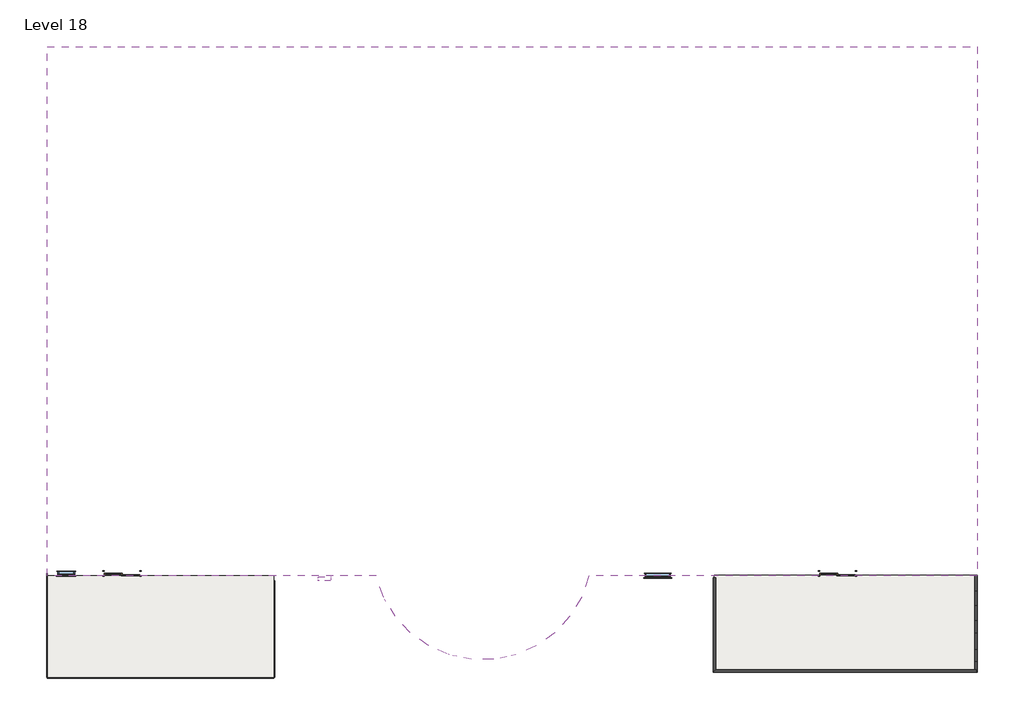
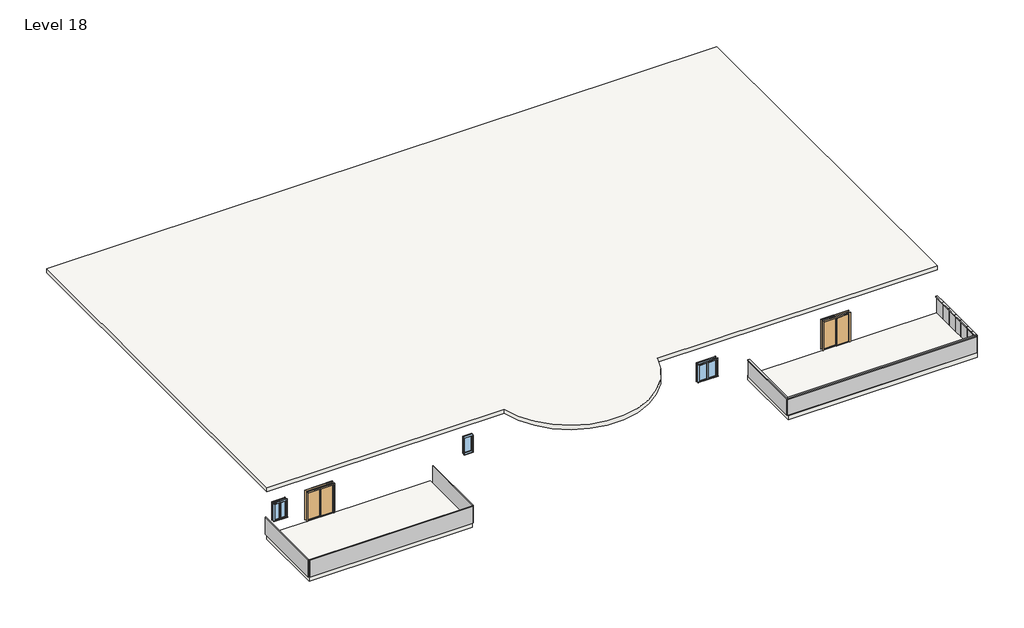
# One storey: 12 plates, 10 members, 3 slabs, 3 windows, 2 doors.
"""IFC4 building model written with IfcOpenShell, lengths in millimetres."""

from ifc_helpers import new_model, si_unit, point, frame, frame_2d, origin, place, context, project, spatial, polyline, circle_curve, trimmed, segment, composite_curve, outline, extrude, transform, mapped, element, save
from components import door_076b30e0, member_47bfaf8a, member_aa870034, member_75074519, member_cae490a4, member_7096a90e, member_cf286210, member_fed80fbc, system_panel_glazed_f269d4c8, system_panel_glazed_7af1c9c3, system_panel_glazed_904ef9a5, system_panel_glazed_078a25c0, system_panel_glazed_c3939aa2, system_panel_glazed_2b5622e6, system_panel_glazed_b96adab1, system_panel_glazed_18441643, system_panel_glazed_400a69f6, window_bb17773d, window_0862ab64, window_80bd9af0

model = new_model("IFC4")

# Units and contexts
model_context = context("Model", 3, world=origin())
ifc_project = project(units=[si_unit("LENGTHUNIT", "METRE", prefix="MILLI")], contexts=[model_context])

# Site, building, storey
site = spatial("IfcSite", under=ifc_project)
building = spatial("IfcBuilding", under=site)
storey = spatial("IfcBuildingStorey", under=building, Name="Level 18", Elevation=29870.4)

# Doors
placement = place(None, origin())
door_shape = door_076b30e0(model_context)
element("IfcDoor", 1, ObjectType="Door-Double-Sliding : 68\" x 80\"", at=placement, inside=storey, context=model_context, shape_type="MappedRepresentation", body=[
    mapped(door_shape, transform((-16191.585279, -12227.7237084, 29870.4), x_axis=(-1.0, 0.0, 0.0), y_axis=(0.0, -1.0, 0.0), z_axis=(0.0, 0.0, 1.0))),
])
element("IfcDoor", 2, ObjectType="Door-Double-Sliding : 68\" x 80\"", at=placement, inside=storey, context=model_context, shape_type="MappedRepresentation", body=[
    mapped(door_shape, transform((18682.614721, -12227.7237084, 29870.4), x_axis=(-1.0, 0.0, 0.0), y_axis=(0.0, -1.0, 0.0), z_axis=(0.0, 0.0, 1.0))),
])

# Members
member_shape = member_47bfaf8a(model_context)
element("IfcMember", 3, ObjectType="Rectangular Mullion : 2.5\" x 5\" rectangular", at=placement, inside=storey, context=model_context, shape_type="MappedRepresentation", body=[
    mapped(member_shape, transform((25445.364721, -15278.1106184, 31089.6), x_axis=(0.0, 0.0, 1.0), y_axis=(-1.0, 0.0, 0.0), z_axis=(0.0, -1.0, 0.0))),
])
element("IfcMember", 4, ObjectType="Rectangular Mullion : 2.5\" x 5\" rectangular", at=placement, inside=storey, context=model_context, shape_type="MappedRepresentation", body=[
    mapped(member_shape, transform((25445.364721, -16649.7106184, 31089.6), x_axis=(0.0, 0.0, 1.0), y_axis=(-1.0, 0.0, 0.0), z_axis=(0.0, -1.0, 0.0))),
])
member_2_shape = member_aa870034(model_context)
element("IfcMember", 5, ObjectType="Rectangular Mullion : 2.5\" x 5\" rectangular", at=placement, inside=storey, context=model_context, shape_type="MappedRepresentation", body=[
    mapped(member_2_shape, transform((25445.364721, -16040.1106184, 31089.6), x_axis=(0.0, 0.0, 1.0), y_axis=(-1.0, 0.0, 0.0), z_axis=(0.0, -1.0, 0.0))),
])
member_3_shape = member_75074519(model_context)
element("IfcMember", 6, ObjectType="Rectangular Mullion : 2.5\" x 5\" rectangular", at=placement, inside=storey, context=model_context, shape_type="MappedRepresentation", body=[
    mapped(member_3_shape, transform((25445.364721, -17106.9106184, 29870.4), x_axis=(0.0, -1.0, 0.0), y_axis=(-1.0, 0.0, 0.0), z_axis=(0.0, 0.0, -1.0))),
])
member_4_shape = member_cae490a4(model_context)
element("IfcMember", 7, ObjectType="Rectangular Mullion : 2.5\" x 5\" rectangular", at=placement, inside=storey, context=model_context, shape_type="MappedRepresentation", body=[
    mapped(member_4_shape, transform((25445.364721, -13193.7193451, 31089.6), x_axis=(0.0, 0.0, 1.0), y_axis=(-1.0, 0.0, 0.0), z_axis=(0.0, -1.0, 0.0))),
])
element("IfcMember", 8, ObjectType="Rectangular Mullion : 2.5\" x 5\" rectangular", at=placement, inside=storey, context=model_context, shape_type="MappedRepresentation", body=[
    mapped(member_4_shape, transform((25445.364721, -13931.1149817, 31089.6), x_axis=(0.0, 0.0, 1.0), y_axis=(-1.0, 0.0, 0.0), z_axis=(0.0, -1.0, 0.0))),
])
element("IfcMember", 9, ObjectType="Rectangular Mullion : 2.5\" x 5\" rectangular", at=placement, inside=storey, context=model_context, shape_type="MappedRepresentation", body=[
    mapped(member_4_shape, transform((25445.364721, -14668.5106184, 31089.6), x_axis=(0.0, 0.0, 1.0), y_axis=(-1.0, 0.0, 0.0), z_axis=(0.0, -1.0, 0.0))),
])
member_5_shape = member_7096a90e(model_context)
element("IfcMember", 10, ObjectType="Rectangular Mullion : 2.5\" x 5\" rectangular", at=placement, inside=storey, context=model_context, shape_type="MappedRepresentation", body=[
    mapped(member_5_shape, transform((25445.364721, -17043.4106184, 31089.6), x_axis=(0.0, 0.0, 1.0), y_axis=(-1.0, 0.0, 0.0), z_axis=(0.0, -1.0, 0.0))),
])
member_6_shape = member_cf286210(model_context)
element("IfcMember", 11, ObjectType="Rectangular Mullion : 2.5\" x 5\" rectangular", at=placement, inside=storey, context=model_context, shape_type="MappedRepresentation", body=[
    mapped(member_6_shape, transform((12687.7364138, -12561.0601244, 31089.6), x_axis=(0.0, 0.0, 1.0), y_axis=(1.0, 0.0, 0.0), z_axis=(0.0, 1.0, 0.0))),
])
member_7_shape = member_fed80fbc(model_context)
element("IfcMember", 12, ObjectType="Rectangular Mullion : 2.5\" x 5\" rectangular", at=placement, inside=storey, context=model_context, shape_type="MappedRepresentation", body=[
    mapped(member_7_shape, transform((12687.7364138, -17106.9106184, 31089.6), x_axis=(0.0, 0.0, 1.0), y_axis=(0.0, 1.0, 0.0), z_axis=(-1.0, 0.0, 0.0))),
])

# Plates
system_panel_glazed_shape = system_panel_glazed_f269d4c8(model_context)
element("IfcPlate", 13, ObjectType="System Panel : Glazed", at=placement, inside=storey, context=model_context, shape_type="MappedRepresentation", body=[
    mapped(system_panel_glazed_shape, transform((25445.364721, -15659.1106184, 29870.4), x_axis=(0.0, -1.0, 0.0), y_axis=(1.0, 0.0, 0.0), z_axis=(0.0, 0.0, 1.0))),
])
system_panel_glazed_2_shape = system_panel_glazed_7af1c9c3(model_context)
element("IfcPlate", 14, ObjectType="System Panel : Glazed", at=placement, inside=storey, context=model_context, shape_type="MappedRepresentation", body=[
    mapped(system_panel_glazed_2_shape, transform((25445.364721, -16344.9106184, 29870.4), x_axis=(0.0, -1.0, 0.0), y_axis=(1.0, 0.0, 0.0), z_axis=(0.0, 0.0, 1.0))),
])
element("IfcPlate", 15, ObjectType="System Panel : Glazed", at=placement, inside=storey, context=model_context, shape_type="MappedRepresentation", body=[
    mapped(system_panel_glazed_2_shape, transform((25445.364721, -14973.3106184, 29870.4), x_axis=(0.0, -1.0, 0.0), y_axis=(1.0, 0.0, 0.0), z_axis=(0.0, 0.0, 1.0))),
])
system_panel_glazed_3_shape = system_panel_glazed_904ef9a5(model_context)
element("IfcPlate", 16, ObjectType="System Panel : Glazed", at=placement, inside=storey, context=model_context, shape_type="MappedRepresentation", body=[
    mapped(system_panel_glazed_3_shape, transform((25445.364721, -12825.0215267, 29870.4), x_axis=(0.0, -1.0, 0.0), y_axis=(1.0, 0.0, 0.0), z_axis=(0.0, 0.0, 1.0))),
])
element("IfcPlate", 17, ObjectType="System Panel : Glazed", at=placement, inside=storey, context=model_context, shape_type="MappedRepresentation", body=[
    mapped(system_panel_glazed_3_shape, transform((25445.364721, -14299.8128001, 29870.4), x_axis=(0.0, -1.0, 0.0), y_axis=(1.0, 0.0, 0.0), z_axis=(0.0, 0.0, 1.0))),
])
element("IfcPlate", 18, ObjectType="System Panel : Glazed", at=placement, inside=storey, context=model_context, shape_type="MappedRepresentation", body=[
    mapped(system_panel_glazed_3_shape, transform((25445.364721, -13562.4171634, 29870.4), x_axis=(0.0, -1.0, 0.0), y_axis=(1.0, 0.0, 0.0), z_axis=(0.0, 0.0, 1.0))),
])
system_panel_glazed_4_shape = system_panel_glazed_078a25c0(model_context)
element("IfcPlate", 19, ObjectType="System Panel : Glazed", at=placement, inside=storey, context=model_context, shape_type="MappedRepresentation", body=[
    mapped(system_panel_glazed_4_shape, transform((19066.5505674, -17106.9106184, 29870.4), x_axis=(-1.0, 0.0, 0.0), y_axis=(0.0, -1.0, 0.0), z_axis=(0.0, 0.0, 1.0))),
])
system_panel_glazed_5_shape = system_panel_glazed_c3939aa2(model_context)
element("IfcPlate", 20, ObjectType="System Panel : Glazed", at=placement, inside=storey, context=model_context, shape_type="MappedRepresentation", body=[
    mapped(system_panel_glazed_5_shape, transform((25445.364721, -16846.5606184, 29870.4), x_axis=(0.0, -1.0, 0.0), y_axis=(1.0, 0.0, 0.0), z_axis=(0.0, 0.0, 1.0))),
])
system_panel_glazed_6_shape = system_panel_glazed_2b5622e6(model_context)
element("IfcPlate", 21, ObjectType="System Panel : Glazed", at=placement, inside=storey, context=model_context, shape_type="MappedRepresentation", body=[
    mapped(system_panel_glazed_6_shape, transform((12687.7364138, -14833.9853714, 29870.4), x_axis=(0.0, 1.0, 0.0), y_axis=(-1.0, 0.0, 0.0), z_axis=(0.0, 0.0, 1.0))),
])
system_panel_glazed_7_shape = system_panel_glazed_b96adab1(model_context)
element("IfcPlate", 22, ObjectType="System Panel : Glazed", at=placement, inside=storey, context=model_context, shape_type="MappedRepresentation", body=[
    mapped(system_panel_glazed_7_shape, transform((-14302.7926538, -17411.944108, 29870.4), x_axis=(-1.0, 0.0, 0.0), y_axis=(0.0, -1.0, 0.0), z_axis=(0.0, 0.0, 1.0))),
])
system_panel_glazed_8_shape = system_panel_glazed_18441643(model_context)
element("IfcPlate", 23, ObjectType="System Panel : Glazed", at=placement, inside=storey, context=model_context, shape_type="MappedRepresentation", body=[
    mapped(system_panel_glazed_8_shape, transform((-19823.785279, -14883.3339082, 29870.4), x_axis=(0.0, 1.0, 0.0), y_axis=(-1.0, 0.0, 0.0), z_axis=(0.0, 0.0, 1.0))),
])
system_panel_glazed_9_shape = system_panel_glazed_400a69f6(model_context)
element("IfcPlate", 24, ObjectType="System Panel : Glazed", at=placement, inside=storey, context=model_context, shape_type="MappedRepresentation", body=[
    mapped(system_panel_glazed_9_shape, transform((-8781.8000285, -15065.3724195, 29870.4), x_axis=(0.0, -1.0, 0.0), y_axis=(1.0, 0.0, 0.0), z_axis=(0.0, 0.0, 1.0))),
])

# Slabs
element("IfcSlab", 25, ObjectType="Generic - 12\"", at=placement, inside=storey, context=model_context, shape_type="SweptSolid", body=[
    extrude(outline(composite_curve([segment(polyline([(25489.814721, 13330.837176), (25489.814721, -12475.562824), (6571.5594464, -12475.562824)]), True, "CONTINUOUS"), segment(trimmed(circle_curve(frame_2d((1385.214721, -11244.9297828)), 5330.3498284), [point((6571.5594464, -12475.562824))], [point((-3801.1300045, -12475.562824))], False, "CARTESIAN"), True, "CONTINUOUS"), segment(polyline([(-3801.1300045, -12475.562824), (-19823.785279, -12475.562824), (-19823.785279, 13330.837176), (25489.814721, 13330.837176)]), True, "CONTINUOUS")], self_intersect=False)), frame((0.0, 0.0, 32956.1464133), z_axis=(0.0, 0.0, 1.0), x_axis=(1.0, 0.0, 0.0)), (0.0, 0.0, 1.0), 304.8),
])
element("IfcSlab", 26, ObjectType="Generic - 12\"", at=placement, inside=storey, context=model_context, shape_type="SweptSolid", body=[
    extrude(outline(polyline([(25489.814721, -12433.6961364), (25489.814721, -17172.4176946), (12687.7364138, -17172.4176946), (12687.7364138, -12433.6961364), (25489.814721, -12433.6961364)])), frame((0.0, 0.0, 29565.6), z_axis=(0.0, 0.0, 1.0), x_axis=(1.0, 0.0, 0.0)), (0.0, 0.0, 1.0), 304.8),
])
element("IfcSlab", 27, ObjectType="Generic - 12\"", at=placement, inside=storey, context=model_context, shape_type="SweptSolid", body=[
    extrude(outline(polyline([(-8781.8000285, -12456.3237084), (-8781.8000285, -17411.944108), (-19823.785279, -17411.944108), (-19823.785279, -12456.3237084), (-8781.8000285, -12456.3237084)])), frame((0.0, 0.0, 29565.6), z_axis=(0.0, 0.0, 1.0), x_axis=(1.0, 0.0, 0.0)), (0.0, 0.0, 1.0), 304.8),
])

# Windows
window_shape = window_bb17773d(model_context)
element("IfcWindow", 28, ObjectType="Casement Dbl with Trim : 32\" x 48\"", at=placement, inside=storey, context=model_context, shape_type="MappedRepresentation", body=[
    mapped(window_shape, transform((-18909.385279, -12335.6737084, 29754.8931655), x_axis=(-1.0, 0.0, 0.0), y_axis=(0.0, -1.0, 0.0), z_axis=(0.0, 0.0, 1.0))),
])
window_2_shape = window_0862ab64(model_context)
element("IfcWindow", 29, ObjectType="Casement Dbl with Trim : 48\" x 48\"", at=placement, inside=storey, context=model_context, shape_type="MappedRepresentation", body=[
    mapped(window_2_shape, transform((9924.3594464, -12437.2737084, 29717.8859618), x_axis=(-1.0, 0.0, 0.0), y_axis=(0.0, -1.0, 0.0), z_axis=(0.0, 0.0, 1.0))),
])
window_3_shape = window_80bd9af0(model_context)
element("IfcWindow", 30, ObjectType="Fixed : 24\" x 48\"", at=placement, inside=storey, context=model_context, shape_type="MappedRepresentation", body=[
    mapped(window_3_shape, transform((-6272.885279, -12617.2007309, 30185.8939938), x_axis=(1.0, 0.0, 0.0), y_axis=(0.0, 1.0, 0.0), z_axis=(0.0, 0.0, 1.0))),
])

save(model, "model.ifc")

# Revit data of these elements
# Type "Door-Double-Sliding : 68\" x 80\""
#   Type Mark = "10"
#   Construction Type Id = "opn-d45"
#   Assembly Code = "C1020"
#   Analytic Construction = "Wood frame, double glass door "
#   Thickness = 0' - 2"
#   Thermal Resistance (R) = 1.8150 (h·ft²·°F)/BTU
#   Heat Transfer Coefficient (U) = 0.5510 BTU/(h·ft²·°F)
#   Height = 6' - 8"
#   Rail Width = 0' - 2"
#   Stiles = 0' - 2"
#   Trim Projection Ext = 0' - 1"
#   Trim Projection Int = 0' - 1"
#   Trim Width = 0' - 3"
#   Width = 5' - 8"
#   Define Thermal Properties by = 1
#   Glazing = Glass
#   Panel Material = Wood - Birch - Solid Stained Light Low Gloss
#   Trim Material = Paint - Sienna
#   Visual Light Transmittance = 0
#   Solar Heat Gain Coefficient = 0
#   Function = (empty or 0)
#   Wall Closure = (empty or 0)
# Type "Rectangular Mullion : 2.5\" x 5\" rectangular"
#   built-in parameter 1007304 = 0.416667 (stored number, unit not read)
#   built-in parameter 1007301 = 0.104167 (stored number, unit not read)
#   built-in parameter 1007300 = 0.104167 (stored number, unit not read)
# Type "System Panel : Glazed"
#   Construction Type Id = "GSP4R"
#   Analytic Construction = "1/8 in Pilkington single glazing"
#   Visual Light Transmittance = 0.9
#   Solar Heat Gain Coefficient = 0.86
#   Heat Transfer Coefficient (U) = 1.18115 BTU/(h·ft²·°F)
# Type "Generic - 12\""
#   Assembly Code = "B1010"
#   Function = 0
#   Layers, outside or top first: 1' - 0" no material (function 1)
# Type "Casement Dbl with Trim : 32\" x 48\""
#   Type Mark = "36"
#   Construction Type Id = "GSP4R"
#   Assembly Code = "B2020100"
#   Analytic Construction = "1/8 in Pilkington single glazing"
#   Visual Light Transmittance = 0.9
#   Solar Heat Gain Coefficient = 0.78
#   Heat Transfer Coefficient (U) = 0.6496 BTU/(h·ft²·°F)
#   Height = 4' - 0"
#   Default Sill Height = 3' - 0"
#   Trim Projection - Ext. = 0' - 0 1/2"
#   Trim Projection - Int. = 0' - 0 3/4"
#   Trim Width - Exterior = 0' - 3 1/2"
#   Trim Width - Interior = 0' - 3 1/2"
#   Width = 2' - 8"
#   Window Inset = 0' - 0 3/4"
#   Define Thermal Properties by = 1
#   Glass Pane Material = Glass
#   Sash Material = Sash
#   Trim Exterior Material = Trim
#   Trim Interior Material = Trim
#   Wall Closure = (empty or 0)
# Type "Casement Dbl with Trim : 48\" x 48\""
#   Type Mark = "34"
#   Construction Type Id = "GSP4R"
#   Assembly Code = "B2020100"
#   Analytic Construction = "1/8 in Pilkington single glazing"
#   Visual Light Transmittance = 0.9
#   Solar Heat Gain Coefficient = 0.78
#   Heat Transfer Coefficient (U) = 0.6496 BTU/(h·ft²·°F)
#   Height = 4' - 0"
#   Default Sill Height = 3' - 0"
#   Trim Projection - Ext. = 0' - 0 1/2"
#   Trim Projection - Int. = 0' - 0 3/4"
#   Trim Width - Exterior = 0' - 3 1/2"
#   Trim Width - Interior = 0' - 3 1/2"
#   Width = 4' - 0"
#   Window Inset = 0' - 0 3/4"
#   Define Thermal Properties by = 1
#   Glass Pane Material = Glass
#   Sash Material = Sash
#   Trim Exterior Material = Trim
#   Trim Interior Material = Trim
#   Wall Closure = (empty or 0)
# Type "Fixed : 24\" x 48\""
#   Type Mark = "2"
#   Construction Type Id = "GSP4R"
#   Assembly Code = "B2020100"
#   Analytic Construction = "1/8 in Pilkington single glazing"
#   Visual Light Transmittance = 0.9
#   Solar Heat Gain Coefficient = 0.78
#   Heat Transfer Coefficient (U) = 0.6496 BTU/(h·ft²·°F)
#   Height = 4' - 0"
#   Default Sill Height = 3' - 0"
#   Width = 2' - 0"
#   Window Inset = 0' - 0 3/4"
#   Define Thermal Properties by = 1
#   Glass Pane Material = Glass
#   Sash Material = Sash
#   Wall Closure = (empty or 0)
# Elements 1, 2 (IfcDoor, "Door-Double-Sliding : 68\" x 80\"")
#   Phase Created = New Construction
#   Materials on its faces: "Paint - Sienna", "Wood - Birch - Solid Stained Light Low Gloss", "Glass"
# Elements 3, 4, 5, 6, 7, 8, 9, 10, 11, 12 (IfcMember, "Rectangular Mullion : 2.5\" x 5\" rectangular")
#   Phase Created = New Construction
#   Materials on its faces: "Aluminum"
# Elements 13, 14, 15, 16, 17, 18, 19, 20, 21, 22, 23, 24 (IfcPlate, "System Panel : Glazed")
#   Phase Created = New Construction
#   Materials on its faces: "Glass"
# Element 25 (IfcSlab, "Generic - 12\"")
#   Height Offset From Level = 11' - 1.48608"
#   Phase Created = New Construction
#   Materials on its faces: "Default Floor"
# Elements 26, 27 (IfcSlab, "Generic - 12\"")
#   Height Offset From Level = 0' - 0"
#   Phase Created = New Construction
#   Materials on its faces: "Default Floor"
# Element 28 (IfcWindow, "Casement Dbl with Trim : 32\" x 48\"")
#   Mark = "42"
#   Phase Created = New Construction
#   Materials on its faces: "Sash", "Trim", "Glass"
# Element 29 (IfcWindow, "Casement Dbl with Trim : 48\" x 48\"")
#   Mark = "8"
#   Phase Created = New Construction
#   Materials on its faces: "Sash", "Trim", "Glass"
# Element 30 (IfcWindow, "Fixed : 24\" x 48\"")
#   Mark = "76"
#   Phase Created = New Construction
#   Materials on its faces: "Sash", "Glass"
# Materials
#   "Glass": class "Glass", colour RGB 0 128 192, transparency 0.75, Description = "Soda Lime Glass", Cost = 0
#   "Wood - Birch - Solid Stained Light Low Gloss": class "Wood", colour RGB 210 159 95, transparency 0, Cost = 0
#   "Paint - Sienna": colour RGB 118 70 51, transparency 0, Cost = 0
#   "Sash": class "Wood", colour RGB 224 178 126, transparency 0
#   "Trim": class "Wood", colour RGB 224 178 126, transparency 0
#   "Aluminum": class "Metal", colour RGB 247 247 247, transparency 0, Description = "Aluminum 6061", Cost = 0
#   "Default Floor": colour RGB 128 128 128, transparency 0
